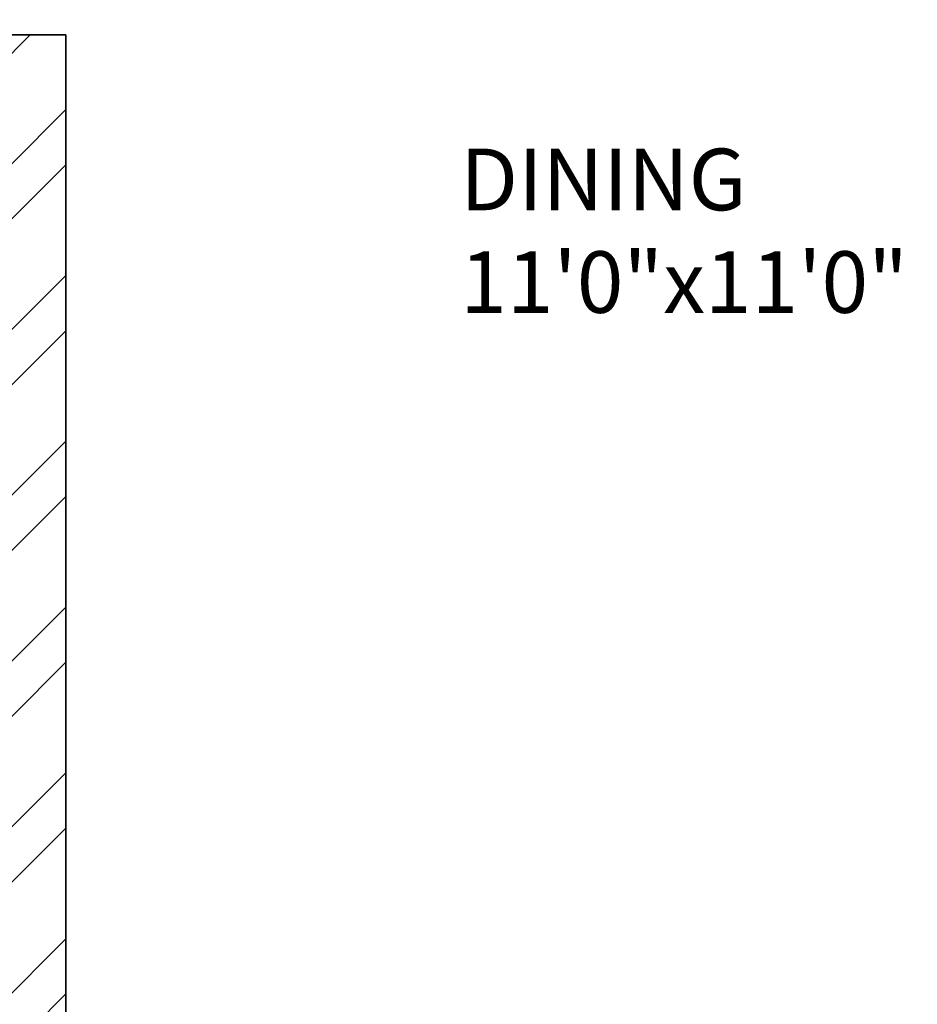
# Model space of a CAD drawing. Units: inches. Extents: x 1962 to 2771, y 1245 to 2660.
# Tile 86 of 114: x 2236 to 2308, y 2180 to 2260. Entities that reach past the tile are written whole.
import ezdxf

# ---------------------------------------------------------------- set-up
doc = ezdxf.new("R2010")
doc.units = ezdxf.units.IN
for name, color, linetype, lineweight in [('A-ANNO-DIMS', 2, 'Continuous', 18), ('A-AREA-IDEN', 7, 'Continuous', 18), ('A-WALL', 7, 'Continuous', 35), ('A-WALL-PATT', 252, 'Continuous', 13)]:
    doc.layers.add(name, color=color, linetype=linetype, lineweight=lineweight)
doc.styles.get("Standard").update_dxf_attribs({"font": 'arial.ttf'})
doc.dimstyles.get("Standard").update_dxf_attribs({"dimtxt": 0.18, "dimasz": 0.18, "dimexe": 0.18, "dimexo": 0.0625, "dimgap": 0.09, "dimtad": 0, "dimtih": 1, "dimtoh": 1, "dimdec": 4, "dimzin": 0, "dimdsep": 46, "dimtxsty": 'Standard', "dimcen": 0.09, "dimadec": 0, "dimazin": 0, "dimtfac": 1, "dimtdec": 4, "dimtofl": 0, "dimtmove": 0, "dimatfit": 3, "dimfxl": 1, "dimtolj": 1, "dimtzin": 0, "dimarcsym": 0})

# ---------------------------------------------------------------- blocks, each defined once
blk = doc.blocks.new('*D40')
at = {"layer": 'A-ANNO-DIMS', "color": 0, "lineweight": -2, "transparency": 16777216}
for p, q in [((2072.02, 2033.906), (2072.02, 2583.474)), ((2072.2, 2583.294), (2366.02, 2583.294)), ((2660.627, 2583.294), (2366.808, 2583.294)), ((2660.807, 2524.406), (2660.807, 2583.474))]:
    blk.add_line(p, q, dxfattribs=at)
at = {"layer": 'A-ANNO-DIMS', "color": 0, "transparency": 16777216}
for points in [[(2072.2, 2583.324), (2072.2, 2583.264), (2072.02, 2583.294)], [(2660.627, 2583.324), (2660.627, 2583.264), (2660.807, 2583.294)]]:
    blk.add_solid(points, dxfattribs=at)
at = {"layer": 'Defpoints', "color": 0, "transparency": 16777216}
for p in [(2660.807, 2583.294), (2660.807, 2524.344), (2072.02, 2033.844)]:
    blk.add_point(p, dxfattribs=at)
at = {"layer": 'A-ANNO-DIMS', "color": 0, "transparency": 16777216, "insert": (2366.414, 2583.294), "char_height": 0.18, "attachment_point": 5}
blk.add_mtext('\\A1;588.8', dxfattribs=at)

msp = doc.modelspace()

# ---------------------------------------------------------------- hatches: boundary and pattern name
at = {"layer": 'A-WALL-PATT'}
h = msp.add_hatch(dxfattribs=at)
h.set_pattern_fill('ANSI32', color=256)
h.paths.add_polyline_path([(2090.8074, 2467.3437), (2141.6481, 2467.3437), (2141.6481, 2469.5937), (2141.6481, 2471.8437), (2086.3074, 2471.8437), (2086.3074, 2422.5333), (2090.8074, 2422.5333)])
h.paths.add_polyline_path([(2282.7664, 2471.8437), (2204.8982, 2471.8437), (2204.8982, 2467.3437), (2234.8074, 2467.3437), (2234.8074, 2311.3437), (2228.7492, 2311.3437), (2228.7492, 2306.8437), (2234.8074, 2306.8437), (2331.9227, 2306.8437), (2331.9227, 2309.0937), (2331.9227, 2311.3437), (2239.3074, 2311.3437), (2239.3074, 2467.3437), (2282.7664, 2467.3437), (2282.7664, 2469.5937)])
h.paths.add_polyline_path([(2471.4531, 2519.8437), (2552.011, 2519.8437), (2564.3996, 2519.8437), (2564.3996, 2511.1389), (2568.8996, 2511.1389), (2568.8996, 2524.3437), (2466.9531, 2524.3437), (2466.9531, 2471.8437), (2450.0749, 2471.8437), (2446.4672, 2471.8437), (2446.4672, 2467.3437), (2450.0749, 2467.3437), (2475.9988, 2467.3437), (2475.9988, 2469.5937), (2475.9988, 2471.8437), (2471.4531, 2471.8437)])
h.paths.add_polyline_path([(2575.2231, 2469.5937), (2575.2231, 2471.8437), (2568.8996, 2471.8437), (2568.8996, 2487.1389), (2564.3996, 2487.1389), (2564.3996, 2471.8437), (2556.511, 2471.8437), (2499.2904, 2471.8437), (2499.2904, 2467.3437), (2507.8074, 2467.3437), (2507.8074, 2311.3437), (2414.863, 2311.3437), (2414.863, 2306.8437), (2512.3074, 2306.8437), (2517.0114, 2306.8437), (2517.0114, 2309.0937), (2517.0114, 2311.3437), (2512.3074, 2311.3437), (2512.3074, 2467.3437), (2575.2231, 2467.3437)])
h.paths.add_polyline_path([(2660.8074, 2471.8437), (2600.9602, 2471.8437), (2600.9602, 2467.3437), (2656.3074, 2467.3437), (2656.3074, 2432.5704), (2660.8074, 2432.5704)])
h.paths.add_polyline_path([(2660.8074, 2372.5704), (2656.3074, 2372.5704), (2656.3074, 2311.3437), (2600.276, 2311.3437), (2600.276, 2309.0937), (2600.276, 2306.8437), (2656.3074, 2306.8437), (2656.3074, 2296.2593), (2660.8074, 2296.2593)])
h.paths.add_polyline_path([(2572.3074, 2306.8437), (2577.1385, 2306.8437), (2577.1385, 2311.3437), (2551.082, 2311.3437), (2551.082, 2306.8437), (2567.8074, 2306.8437), (2567.8074, 2258.8437), (2540.0574, 2258.8437), (2540.0574, 2256.5937), (2540.0574, 2254.3437), (2567.8074, 2254.3437), (2656.3074, 2254.3437), (2656.3074, 2236.9085), (2660.8074, 2236.9085), (2660.8074, 2272.2593), (2656.3074, 2272.2593), (2656.3074, 2258.8437), (2572.3074, 2258.8437)])
h.paths.add_polyline_path([(2512.3074, 2254.3437), (2518.8716, 2254.3437), (2518.8716, 2256.5937), (2518.8716, 2258.8437), (2507.8074, 2258.8437), (2507.8074, 2177.8437), (2567.8074, 2177.8437), (2567.8074, 2172.9628), (2572.3074, 2172.9628), (2572.3074, 2177.8437), (2656.3074, 2177.8437), (2656.3074, 2166.4846), (2660.8074, 2166.4846), (2660.8074, 2200.9085), (2656.3074, 2200.9085), (2656.3074, 2182.3437), (2512.3074, 2182.3437)])
h.paths.add_polyline_path([(2656.3074, 2129.8437), (2572.3074, 2129.8437), (2572.3074, 2150.3044), (2570.0574, 2150.3044), (2567.8074, 2150.3044), (2567.8074, 2129.8437), (2507.8074, 2129.8437), (2507.8074, 2116.3027), (2510.0574, 2116.3027), (2512.3074, 2116.3027), (2512.3074, 2125.3437), (2567.8074, 2125.3437), (2572.3074, 2125.3437), (2656.3074, 2125.3437)])
h.paths.add_polyline_path([(2090.8074, 2362.5333), (2086.3074, 2362.5333), (2086.3074, 2298.6242), (2090.8074, 2298.6242), (2090.8074, 2306.8437), (2174.8074, 2306.8437), (2174.8074, 2286.4178), (2179.3074, 2286.4178), (2179.3074, 2306.8437), (2192.8641, 2306.8437), (2192.8641, 2309.0937), (2192.8641, 2311.3437), (2090.8074, 2311.3437)])
h.paths.add_polyline_path([(2209.156, 2258.8437), (2179.3074, 2258.8437), (2179.3074, 2263.2236), (2177.0574, 2263.2236), (2174.8074, 2263.2236), (2174.8074, 2258.8437), (2090.8074, 2258.8437), (2090.8074, 2274.6242), (2086.3074, 2274.6242), (2086.3074, 2238.2967), (2088.5574, 2238.2967), (2090.8074, 2238.2967), (2090.8074, 2254.3437), (2209.156, 2254.3437)])
h.paths.add_polyline_path([(2090.8074, 2177.8437), (2234.8074, 2177.8437), (2234.8074, 2173.1428), (2239.3074, 2173.1428), (2239.3074, 2258.8437), (2230.8442, 2258.8437), (2230.8442, 2256.5937), (2230.8442, 2254.3437), (2234.8074, 2254.3437), (2234.8074, 2182.3437), (2090.8074, 2182.3437), (2090.8074, 2202.2967), (2086.3074, 2202.2967), (2086.3074, 2140.0389), (2090.8074, 2140.0389)])
h.paths.add_polyline_path([(2090.8074, 2080.0389), (2086.3074, 2080.0389), (2086.3074, 2033.8437), (2090.8074, 2033.8437)], flags=17)
h.paths.add_polyline_path([(2244.9405, 2033.8437), (2239.3074, 2033.8437), (2239.3074, 2142.0665), (2237.2592, 2142.0665), (2234.8074, 2142.0665), (2234.8074, 2033.8437), (2090.8074, 2033.8437), (2076.5204, 2033.8437), (2072.0204, 2033.8437), (2072.0204, 2000.4493), (2076.5204, 2000.4493), (2076.5204, 2029.3437), (2090.8074, 2029.3437), (2244.9405, 2029.3437), (2244.9405, 2031.5937)])
h.paths.add_polyline_path([(2234.8074, 1933.3437), (2076.5204, 1933.3437), (2076.5204, 1952.4493), (2074.2704, 1952.4493), (2072.0204, 1952.4493), (2072.0204, 1933.3437), (2072.0204, 1928.8437), (2234.8074, 1928.8437)])
h.paths.add_polyline_path([(2090.8074, 1928.8437), (2086.3074, 1928.8437), (2086.3074, 1906.5013), (2090.8074, 1906.5013)])
h.paths.add_polyline_path([(2090.8074, 1846.5013), (2086.3074, 1846.5013), (2086.3074, 1769.9917), (2088.5574, 1769.9917), (2090.8074, 1769.9917), (2090.8074, 1780.3437), (2234.8074, 1780.3437), (2234.8074, 1708.3437), (2230.3764, 1708.3437), (2230.3764, 1703.8437), (2239.3074, 1703.8437), (2239.3074, 1792.6669), (2237.0574, 1792.6669), (2234.8074, 1792.6669), (2234.8074, 1784.8437), (2090.8074, 1784.8437)])
h.paths.add_polyline_path([(2239.3074, 1928.8437), (2244.9405, 1928.8437), (2244.9405, 1931.0937), (2244.9405, 1933.3437), (2234.8074, 1933.3437), (2234.8074, 1928.8437), (2234.8074, 1825.5949), (2239.3074, 1825.5949)])
h.paths.add_polyline_path([(2148.0425, 1649.0937), (2148.0425, 1651.3437), (2090.8074, 1651.3437), (2090.8074, 1646.8437), (2148.0425, 1646.8437)], flags=0)
h.paths.add_polyline_path([(2207.5601, 1708.3437), (2090.8074, 1708.3437), (2090.8074, 1703.8437), (2174.8074, 1703.8437), (2174.8074, 1651.3437), (2170.4457, 1651.3437), (2170.4457, 1646.8437), (2195.9924, 1646.8437), (2195.9924, 1649.0937), (2195.9924, 1651.3437), (2179.3074, 1651.3437), (2179.3074, 1703.8437), (2207.5601, 1703.8437), (2207.5601, 1706.0937)])
h.paths.add_polyline_path([(2090.8074, 1733.9917), (2086.3074, 1733.9917), (2086.3074, 1696.1032), (2088.5574, 1696.1032), (2090.8074, 1696.1032)])
h.paths.add_polyline_path([(2090.8074, 1672.1032), (2086.3074, 1672.1032), (2086.3074, 1600.3335), (2090.8074, 1600.3335)])
h.paths.add_polyline_path([(2090.8074, 1540.3335), (2086.3074, 1540.3335), (2086.3074, 1486.3437), (2139.6766, 1486.3437), (2139.6766, 1490.8437), (2090.8074, 1490.8437)])
h.paths.add_polyline_path([(2302.3876, 1490.8437), (2239.3074, 1490.8437), (2239.3074, 1646.8437), (2335.9994, 1646.8437), (2335.9994, 1651.3437), (2229.884, 1651.3437), (2229.884, 1646.8437), (2234.8074, 1646.8437), (2234.8074, 1490.8437), (2202.7103, 1490.8437), (2202.7103, 1488.5937), (2202.7103, 1486.3437), (2275.0699, 1486.3437), (2275.0699, 1475.772), (2279.5699, 1475.772), (2279.5699, 1486.3437), (2302.3876, 1486.3437)])
h.paths.add_polyline_path([(2279.5699, 1451.772), (2275.0699, 1451.772), (2275.0699, 1438.3437), (2174.8074, 1438.3437), (2174.8074, 1486.3437), (2179.7922, 1486.3437), (2179.7922, 1490.8437), (2163.3585, 1490.8437), (2163.3585, 1488.5937), (2163.3585, 1486.3437), (2170.3074, 1486.3437), (2170.3074, 1433.8437), (2279.5699, 1433.8437)])
h.paths.add_polyline_path([(2427.2363, 1490.8437), (2375.8074, 1490.8437), (2375.8074, 1646.8437), (2381.6401, 1646.8437), (2381.6401, 1651.3437), (2365.887, 1651.3437), (2365.887, 1649.0937), (2365.887, 1646.8437), (2371.3074, 1646.8437), (2371.3074, 1490.8437), (2327.5627, 1490.8437), (2327.5627, 1488.5937), (2327.5627, 1486.3437), (2371.3074, 1486.3437), (2371.3074, 1433.8437), (2375.8074, 1433.8437), (2375.8074, 1486.3437), (2427.2363, 1486.3437)])
h.paths.add_polyline_path([(2512.3074, 1646.8437), (2519.4351, 1646.8437), (2519.4351, 1649.0937), (2519.4351, 1651.3437), (2507.8074, 1651.3437), (2416.0063, 1651.3437), (2416.0063, 1649.0937), (2416.0063, 1646.8437), (2507.8074, 1646.8437), (2507.8074, 1490.8437), (2497.0532, 1490.8437), (2497.0532, 1488.5937), (2497.0532, 1486.3437), (2574.9344, 1486.3437), (2574.9344, 1476.0181), (2579.4344, 1476.0181), (2579.4344, 1486.3437), (2584.4872, 1486.3437), (2584.3074, 1490.8437), (2512.3074, 1490.8437)])
h.paths.add_polyline_path([(2470.5091, 1486.3437), (2473.9767, 1486.3437), (2473.9767, 1490.8437), (2449.6605, 1490.8437), (2449.6605, 1488.5937), (2449.6605, 1486.3437), (2466.0091, 1486.3437), (2466.0091, 1433.8437), (2470.5091, 1433.8437), (2579.4344, 1433.8437), (2579.4344, 1452.0181), (2574.9344, 1452.0181), (2574.9344, 1438.3437), (2554.5091, 1438.3437), (2470.5091, 1438.3437)])
h.paths.add_polyline_path([(2656.3074, 1490.8437), (2611.86, 1490.8437), (2611.86, 1486.3437), (2656.3074, 1486.3437)])
h.paths.add_polyline_path([(2660.8074, 1532.7007), (2658.5574, 1532.7007), (2656.3074, 1532.7007), (2656.3074, 1486.3437), (2660.8074, 1486.3437)])
h.paths.add_polyline_path([(2660.8074, 1664.9663), (2656.3074, 1664.9663), (2656.3074, 1651.3437), (2602.2313, 1651.3437), (2602.2313, 1646.8437), (2656.3074, 1646.8437), (2656.3074, 1592.7007), (2660.8074, 1592.7007)])
h.paths.add_polyline_path([(2660.8074, 1724.5221), (2656.3074, 1724.5221), (2656.3074, 1703.8437), (2542.4725, 1703.8437), (2542.4725, 1699.3437), (2567.8074, 1699.3437), (2567.8074, 1651.3437), (2552.7766, 1651.3437), (2552.7766, 1649.0937), (2552.7766, 1646.8437), (2577.2878, 1646.8437), (2577.2878, 1649.0937), (2577.2878, 1651.3437), (2572.3074, 1651.3437), (2572.3074, 1699.3437), (2656.3074, 1699.3437), (2656.3074, 1688.9663), (2660.8074, 1688.9663)])
h.paths.add_polyline_path([(2660.8074, 1880.6524), (2656.3074, 1880.6524), (2656.3074, 1832.8437), (2512.3074, 1832.8437), (2512.3074, 1837.8959), (2507.8074, 1837.8959), (2507.8074, 1828.3437), (2567.8074, 1828.3437), (2567.8074, 1804.3437), (2572.3074, 1804.3437), (2572.3074, 1828.3437), (2656.3074, 1828.3437), (2656.3074, 1818.6778), (2660.8074, 1818.6778)])
h.paths.add_polyline_path([(2660.8074, 1794.6778), (2656.3074, 1794.6778), (2656.3074, 1780.3437), (2572.3074, 1780.3437), (2572.3074, 1783.0303), (2570.0574, 1783.0303), (2567.8074, 1783.0303), (2567.8074, 1780.3437), (2507.8074, 1780.3437), (2507.8074, 1699.3437), (2517.8858, 1699.3437), (2517.8858, 1701.5937), (2517.8858, 1703.8437), (2512.3074, 1703.8437), (2512.3074, 1775.8437), (2656.3074, 1775.8437), (2656.3074, 1760.5221), (2660.8074, 1760.5221)])
h.paths.add_polyline_path([(2660.8074, 1981.3437), (2660.8074, 2020.2808), (2658.5574, 2020.2808), (2656.3074, 2020.2808), (2656.3074, 1981.3437), (2512.3074, 1981.3437), (2512.3074, 2086.6996), (2507.8074, 2086.6996), (2507.8074, 1981.3437), (2375.8074, 1981.3437), (2375.8074, 1986.8505), (2373.5574, 1986.8505), (2371.3074, 1986.8505), (2371.3074, 1973.2607), (2375.8074, 1973.2607), (2375.8074, 1976.8437), (2507.8074, 1976.8437), (2507.8074, 1865.4281), (2510.0574, 1865.4281), (2512.3074, 1865.4281), (2512.3074, 1976.8437), (2660.8074, 1976.8437)])
h.paths.add_polyline_path([(2375.8074, 1940.297), (2373.5574, 1940.297), (2371.3074, 1940.297), (2371.3074, 1933.3437), (2278.4434, 1933.3437), (2278.4434, 1928.8437), (2371.3074, 1928.8437), (2371.3074, 1651.3437), (2375.8074, 1651.3437)])
h.paths.add_polyline_path([(2660.8074, 1976.8437), (2656.3074, 1976.8437), (2656.3074, 1940.6524), (2660.8074, 1940.6524)], flags=17)
h.paths.add_polyline_path([(2660.8074, 2142.4846), (2656.3074, 2142.4846), (2656.3074, 2080.2808), (2660.8074, 2080.2808)])
h.paths.add_polyline_path([(2381.4189, 2311.3437), (2375.8074, 2311.3437), (2375.8074, 2467.3437), (2424.7242, 2467.3437), (2424.7242, 2469.5937), (2424.7242, 2471.8437), (2375.8074, 2471.8437), (2375.8074, 2524.3437), (2371.3074, 2524.3437), (2371.3074, 2471.8437), (2307.2097, 2471.8437), (2307.2097, 2467.3437), (2371.3074, 2467.3437), (2371.3074, 2311.3437), (2366.8901, 2311.3437), (2366.8901, 2306.8437), (2371.3074, 2306.8437), (2371.3074, 2033.8437), (2279.6589, 2033.8437), (2279.6589, 2029.3437), (2371.3074, 2029.3437), (2371.3074, 2014.2598), (2375.8074, 2014.2598), (2375.8074, 2306.8437), (2381.4189, 2306.8437)])
h.paths.add_polyline_path([(2263.3074, 2524.3437), (2170.3074, 2524.3437), (2170.3074, 2519.8437), (2170.3074, 2471.8437), (2165.0312, 2471.8437), (2165.0312, 2467.3437), (2179.6721, 2467.3437), (2179.6721, 2469.5161), (2179.6721, 2471.8437), (2174.8074, 2471.8437), (2174.8074, 2519.8437), (2258.8074, 2519.8437), (2258.8074, 2511.6436), (2263.3074, 2511.6436)])
h.paths.add_polyline_path([(2245.0232, 1361.4123), (2492.9468, 1361.4123), (2492.9468, 1398.505), (2245.0232, 1398.505)], flags=9)
h.paths.add_polyline_path([(2388.1434, 2086.6936), (2425.0704, 2086.6936), (2425.0704, 2105.3509), (2388.1434, 2105.3509)], flags=9)
h.paths.add_polyline_path([(2404.922, 2242.6744), (2445.7337, 2242.6744), (2445.7337, 2261.3318), (2404.922, 2261.3318)], flags=9)
h.paths.add_polyline_path([(2269.4107, 2156.7935), (2306.3378, 2156.7935), (2306.3378, 2175.4508), (2269.4107, 2175.4508)], flags=9)
h.paths.add_polyline_path([(2269.3277, 2233.4343), (2306.2547, 2233.4343), (2306.2547, 2252.0917), (2269.3277, 2252.0917)], flags=9)
h.paths.add_polyline_path([(2431.6052, 2320.6922), (2470.4456, 2320.6922), (2470.4456, 2339.3495), (2431.6052, 2339.3495)], flags=25)
h.paths.add_polyline_path([(2249.6902, 2315.7608), (2288.5306, 2315.7608), (2288.5306, 2334.4182), (2249.6902, 2334.4182)], flags=25)
h.paths.add_polyline_path([(2096.9301, 2314.3181), (2135.7704, 2314.3181), (2135.7704, 2332.9755), (2096.9301, 2332.9755)], flags=25)
h.paths.add_polyline_path([(2134.3475, 2285.7089), (2161.4655, 2285.7089), (2161.4655, 2304.3662), (2134.3475, 2304.3662)], flags=9)
h.paths.add_polyline_path([(2126.5155, 2209.4076), (2159.9227, 2209.4076), (2159.9227, 2228.065), (2126.5155, 2228.065)], flags=25)
h.paths.add_polyline_path([(2110.5753, 2141.5299), (2149.4157, 2141.5299), (2149.4157, 2160.1872), (2110.5753, 2160.1872)], flags=25)
h.paths.add_polyline_path([(2249.8618, 1968.3317), (2286.3966, 1968.3317), (2286.3966, 1986.989), (2249.8618, 1986.989)], flags=9)
h.paths.add_polyline_path([(2395.9507, 1777.0051), (2436.7624, 1777.0051), (2436.7624, 1795.6625), (2395.9507, 1795.6625)], flags=9)
h.paths.add_polyline_path([(2398.5259, 1888.5651), (2435.0062, 1888.5651), (2435.0062, 1907.2224), (2398.5259, 1907.2224)], flags=25)
h.paths.add_polyline_path([(2259.3506, 1728.3559), (2296.2776, 1728.3559), (2296.2776, 1747.0132), (2259.3506, 1747.0132)], flags=9)
h.paths.add_polyline_path([(2271.3698, 1845.268), (2308.2968, 1845.268), (2308.2968, 1863.9253), (2271.3698, 1863.9253)], flags=9)
h.paths.add_polyline_path([(2120.9355, 1786.3027), (2159.7759, 1786.3027), (2159.7759, 1804.9601), (2120.9355, 1804.9601)], flags=25)
h.paths.add_polyline_path([(2121.3164, 1732.1043), (2154.7236, 1732.1043), (2154.7236, 1750.7616), (2121.3164, 1750.7616)], flags=25)
h.paths.add_polyline_path([(2118.3706, 1678.8997), (2147.5282, 1678.8997), (2147.5282, 1697.557), (2118.3706, 1697.557)], flags=25)
h.paths.add_polyline_path([(2385.9227, 1493.557), (2424.763, 1493.557), (2424.763, 1512.2143), (2385.9227, 1512.2143)], flags=25)
h.paths.add_polyline_path([(2248.7058, 1500.0256), (2287.5462, 1500.0256), (2287.5462, 1518.6829), (2248.7058, 1518.6829)], flags=25)
h.paths.add_polyline_path([(2104.1669, 1617.3771), (2143.0073, 1617.3771), (2143.0073, 1636.0344), (2104.1669, 1636.0344)], flags=9)
h.paths.add_polyline_path([(2096.0714, 1447.8824), (2137.3845, 1447.8824), (2137.3845, 1458.1859), (2096.0714, 1458.1859)], flags=9)
h.paths.add_polyline_path([(2180.6114, 1440.325), (2209.7689, 1440.325), (2209.7689, 1458.9823), (2180.6114, 1458.9823)], flags=25)
h.paths.add_polyline_path([(2316.1698, 1447.9637), (2357.4829, 1447.9637), (2357.4829, 1458.2673), (2316.1698, 1458.2673)], flags=9)
h.paths.add_polyline_path([(2397.6187, 1447.9637), (2438.9318, 1447.9637), (2438.9318, 1458.2673), (2397.6187, 1458.2673)], flags=9)
h.paths.add_polyline_path([(2473.0778, 1439.5953), (2502.2354, 1439.5953), (2502.2354, 1458.2527), (2473.0778, 1458.2527)], flags=25)
h.paths.add_polyline_path([(2589.7027, 1447.8819), (2631.0158, 1447.8819), (2631.0158, 1458.1855), (2589.7027, 1458.1855)], flags=9)
h.paths.add_polyline_path([(2522.4009, 1497.5285), (2561.2413, 1497.5285), (2561.2413, 1516.1859), (2522.4009, 1516.1859)], flags=25)
h.paths.add_polyline_path([(2579.6565, 1671.3482), (2608.8141, 1671.3482), (2608.8141, 1690.0056), (2579.6565, 1690.0056)], flags=25)
h.paths.add_polyline_path([(2544.7038, 1725.5064), (2578.1111, 1725.5064), (2578.1111, 1744.1637), (2544.7038, 1744.1637)], flags=25)
h.paths.add_polyline_path([(2578.1191, 1807.472), (2607.2766, 1807.472), (2607.2766, 1826.1293), (2578.1191, 1826.1293)], flags=25)
h.paths.add_polyline_path([(2595.0614, 1835.1839), (2633.9018, 1835.1839), (2633.9018, 1853.8413), (2595.0614, 1853.8413)], flags=25)
h.paths.add_polyline_path([(2567.0097, 2097.7035), (2605.8501, 2097.7035), (2605.8501, 2116.3609), (2567.0097, 2116.3609)], flags=9)
h.paths.add_polyline_path([(2586.644, 2134.6454), (2615.8015, 2134.6454), (2615.8015, 2153.3027), (2586.644, 2153.3027)], flags=9)
h.paths.add_polyline_path([(2544.6185, 2212.6783), (2578.0258, 2212.6783), (2578.0258, 2231.3356), (2544.6185, 2231.3356)], flags=25)
h.paths.add_polyline_path([(2577.0273, 2256.9023), (2606.1849, 2256.9023), (2606.1849, 2275.5597), (2577.0273, 2275.5597)], flags=24)
h.paths.add_polyline_path([(2605.2683, 2315.2821), (2644.1087, 2315.2821), (2644.1087, 2333.9395), (2605.2683, 2333.9395)], flags=25)
h.paths.add_polyline_path([(2583.1244, 2496.1815), (2624.4375, 2496.1815), (2624.4375, 2506.4851), (2583.1244, 2506.4851)], flags=9)
h.paths.add_polyline_path([(2474.761, 2497.0823), (2503.9185, 2497.0823), (2503.9185, 2515.7397), (2474.761, 2515.7397)], flags=25)
h.paths.add_polyline_path([(2387.5787, 2494.2563), (2428.902, 2494.2563), (2428.902, 2504.5598), (2387.5787, 2504.5598)], flags=9)
h.paths.add_polyline_path([(2300.1657, 2500.1564), (2341.4788, 2500.1564), (2341.4788, 2510.46), (2300.1657, 2510.46)], flags=25)
h.paths.add_polyline_path([(2176.8589, 2497.5843), (2206.0165, 2497.5843), (2206.0165, 2516.2416), (2176.8589, 2516.2416)], flags=25)
h.paths.add_polyline_path([(2097.4668, 2494.9762), (2138.7799, 2494.9762), (2138.7799, 2505.2798), (2097.4668, 2505.2798)], flags=9)

# ---------------------------------------------------------------- linework, layer by layer
at = {"layer": 'A-WALL'}
for p, q in [((2230.8442, 2258.8437), (2239.3074, 2258.8437)), ((2239.3074, 2258.8437), (2239.3074, 2173.1428))]:
    msp.add_line(p, q, dxfattribs=at)

# ---------------------------------------------------------------- texts
at = {"layer": 'A-AREA-IDEN', "insert": (2271.3382, 2249.6036), "char_height": 5, "attachment_point": 1}
msp.add_mtext_dynamic_manual_height_columns('DINING\\P11\'0"x11\'0"', width=197.701544, gutter_width=12.5, heights=[0], dxfattribs=at)

# ---------------------------------------------------------------- dimensions: what is measured, and where the dimension line sits
at = {"layer": 'A-ANNO-DIMS'}
dim = msp.add_linear_dim(base=(2660.8074, 2583.2937), p1=(2072.0204, 2033.8437), p2=(2660.8074, 2524.3437), dimstyle='Standard', override={"dimdec": 1, "dimlfac": 1, "dimrnd": 0, "dimzin": 0, "dimdsep": 46, "dimlunit": 2}, dxfattribs=at)
dim.commit()
dim.dimension.update_dxf_attribs({"geometry": '*D40', "text_midpoint": (2366.4139, 2583.2937)})

doc.saveas('drawing.dxf')
